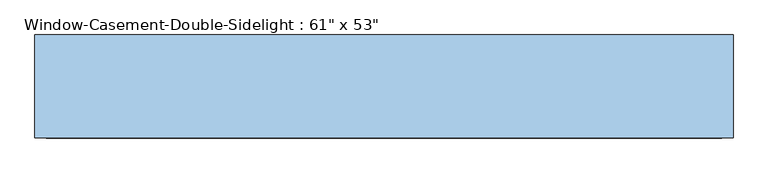
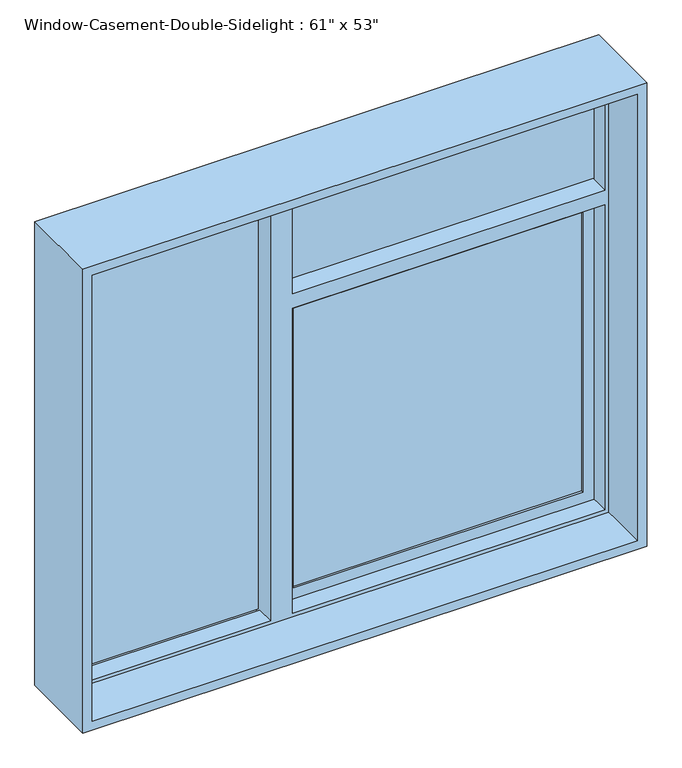
"""IFC4 building model written with IfcOpenShell, lengths in millimetres: window geometry."""

from ifc_helpers import new_model, si_unit, frame, origin, place, context, project, spatial, polyline, outline, extrude, faceted_brep, source, transform, mapped, element, save


def window_390faff0(model_context):
    return source(origin(), model_context, "Body", "SolidModel", [
        extrude(outline(polyline([(707.4296875, 98.425), (-87.6696875, 98.425), (-87.6696875, 111.125), (707.4296875, 111.125), (707.4296875, 98.425)])), frame((0.0, 0.0, 981.6703125), z_axis=(0.0, 0.0, 1.0), x_axis=(1.0, 0.0, 0.0)), (0.0, 0.0, 1.0), 812.2642187),
        extrude(outline(polyline([(707.4296875, 85.725), (707.4296875, 79.375), (-87.6696875, 79.375), (-87.6696875, 85.725), (707.4296875, 85.725)])), frame((0.0, 0.0, 981.6703125), z_axis=(0.0, 0.0, 1.0), x_axis=(1.0, 0.0, 0.0)), (0.0, 0.0, 1.0), 812.2642187),
        extrude(outline(polyline([(-180.34, 98.425), (-180.34, 92.075), (-749.3, 92.075), (-749.3, 98.425), (-180.34, 98.425)])), frame((0.0, 0.0, 949.9203125), z_axis=(0.0, 0.0, 1.0), x_axis=(1.0, 0.0, 0.0)), (0.0, 0.0, 1.0), 1285.2796875),
        extrude(outline(polyline([(-180.34, 85.725), (-180.34, 79.375), (-749.3, 79.375), (-749.3, 85.725), (-180.34, 85.725)])), frame((0.0, 0.0, 949.9203125), z_axis=(0.0, 0.0, 1.0), x_axis=(1.0, 0.0, 0.0)), (0.0, 0.0, 1.0), 1285.2796875),
        extrude(outline(polyline([(749.3, 85.725), (749.3, 79.375), (-129.54, 79.375), (-129.54, 85.725), (749.3, 85.725)])), frame((0.0, 0.0, 1877.6751563), z_axis=(0.0, 0.0, 1.0), x_axis=(1.0, 0.0, 0.0)), (0.0, 0.0, 1.0), 357.5248438),
        extrude(outline(polyline([(749.3, 98.425), (749.3, 92.075), (-129.54, 92.075), (-129.54, 98.425), (749.3, 98.425)])), frame((0.0, 0.0, 1877.6751563), z_axis=(0.0, 0.0, 1.0), x_axis=(1.0, 0.0, 0.0)), (0.0, 0.0, 1.0), 357.5248438),
        faceted_brep([(-749.3, 73.025, 2235.2), (-749.3, 114.3, 2235.2), (749.3, 114.3, 2235.2), (749.3, 73.025, 2235.2), (-129.54, 73.025, 2235.2), (-129.54, 111.125, 2235.2), (-180.34, 111.125, 2235.2), (-180.34, 73.025, 2235.2), (-739.1796875, 22.225, 2225.0796875), (-739.1796875, 73.025, 2225.0796875), (-180.34, 73.025, 2225.0796875), (-180.34, 22.225, 2225.0796875), (739.1796875, 73.025, 2225.0796875), (739.1796875, 22.225, 2225.0796875), (-119.4196875, 22.225, 2225.0796875), (-119.4196875, 73.025, 2225.0796875), (-749.3, -114.3, 2235.2), (-749.3, 22.225, 2235.2), (749.3, 22.225, 2235.2), (749.3, -114.3, 2235.2), (-774.7, 114.3, 2260.6), (-774.7, -114.3, 2260.6), (774.7, -114.3, 2260.6), (774.7, 114.3, 2260.6), (749.3, 114.3, 939.8), (749.3, 73.025, 939.8), (749.3, 73.025, 1835.8048438), (749.3, 111.125, 1835.8048438), (749.3, 111.125, 1877.6751563), (749.3, 73.025, 1877.6751563), (739.1796875, 73.025, 1877.6751563), (739.1796875, 22.225, 1877.6751563), (739.1796875, 73.025, 949.9203125), (739.1796875, 22.225, 949.9203125), (739.1796875, 22.225, 1835.8048438), (739.1796875, 73.025, 1835.8048438), (749.3, 22.225, 939.8), (749.3, -114.3, 939.8), (774.7, -114.3, 914.4), (774.7, 114.3, 914.4), (-749.3, 114.3, 939.8), (-749.3, 73.025, 939.8), (-180.34, 73.025, 939.8), (-180.34, 111.125, 939.8), (-129.54, 111.125, 939.8), (-129.54, 73.025, 939.8), (-119.4196875, 73.025, 949.9203125), (-119.4196875, 22.225, 949.9203125), (-739.1796875, 73.025, 949.9203125), (-739.1796875, 22.225, 949.9203125), (-180.34, 22.225, 949.9203125), (-180.34, 73.025, 949.9203125), (-749.3, 22.225, 939.8), (-749.3, -114.3, 939.8), (-774.7, -114.3, 914.4), (-774.7, 114.3, 914.4), (-119.4196875, 73.025, 1877.6751563), (-129.54, 73.025, 1877.6751563), (-129.54, 73.025, 1835.8048438), (-119.4196875, 73.025, 1835.8048438), (-119.4196875, 22.225, 1877.6751563), (-119.4196875, 22.225, 1835.8048438), (-129.54, 111.125, 1877.6751563), (-129.54, 111.125, 1835.8048438)], [[[0, 1, 2, 3, 4, 5, 6, 7]], [[8, 9, 10, 11]], [[12, 13, 14, 15]], [[16, 17, 18, 19]], [[20, 21, 22, 23]], [[3, 2, 24, 25, 26, 27, 28, 29]], [[13, 12, 30, 31]], [[32, 33, 34, 35]], [[19, 18, 36, 37]], [[23, 22, 38, 39]], [[25, 24, 40, 41, 42, 43, 44, 45]], [[33, 32, 46, 47]], [[48, 49, 50, 51]], [[37, 36, 52, 53]], [[39, 38, 54, 55]], [[1, 0, 41, 40]], [[12, 15, 56, 57, 4, 3, 29, 30]], [[46, 32, 35, 26, 25, 45, 58, 59]], [[41, 0, 7, 10, 9, 48, 51, 42]], [[9, 8, 49, 48]], [[17, 52, 36, 18], [13, 31, 60, 14], [33, 47, 61, 34], [49, 8, 11, 50]], [[17, 16, 53, 52]], [[22, 21, 54, 38], [16, 19, 37, 53]], [[21, 20, 55, 54]], [[20, 23, 39, 55], [2, 1, 40, 24]], [[43, 6, 5, 62, 28, 27, 63, 44]], [[6, 43, 42, 51, 50, 11, 10, 7]], [[15, 14, 60, 56]], [[47, 46, 59, 61]], [[5, 4, 57, 62]], [[45, 44, 63, 58]], [[63, 27, 26, 35, 34, 61, 59, 58]], [[28, 62, 57, 56, 60, 31, 30, 29]]]),
        extrude(outline(polyline([(1835.8048438, 749.3), (1835.8048438, -129.54), (939.8, -129.54), (939.8, 749.3), (1835.8048438, 749.3)]), holes=[polyline([(981.6703125, 707.4296875), (981.6703125, -87.6696875), (1793.9345313, -87.6696875), (1793.9345313, 707.4296875), (981.6703125, 707.4296875)])]), frame((0.0, 73.025, 0.0), z_axis=(0.0, 1.0, 0.0), x_axis=(0.0, 0.0, 1.0)), (0.0, 0.0, 1.0), 31.75),
    ])


if __name__ == "__main__":
    model = new_model("IFC4")
    model_context = context("Model", 3, world=origin())
    ifc_project = project(units=[si_unit("LENGTHUNIT", "METRE", prefix="MILLI")], contexts=[model_context])
    site = spatial("IfcSite", under=ifc_project)
    building = spatial("IfcBuilding", under=site)
    placement = place(None, origin())
    window_shape = window_390faff0(model_context)
    element("IfcWindow", 1, ObjectType="Window-Casement-Double-Sidelight : 61\" x 53\"", at=placement, inside=building, context=model_context, shape_type="MappedRepresentation", body=[
        mapped(window_shape, transform((0.0, 0.0, 0.0), x_axis=(1.0, 0.0, 0.0), y_axis=(0.0, 1.0, 0.0), z_axis=(0.0, 0.0, 1.0))),
    ])
    save(model, "model.ifc")

# Revit data of these elements
# Type "Window-Casement-Double-Sidelight : 61\" x 53\""
#   Type Mark = "21"
#   Fire Rating = "0.5h"
#   Assembly Code = "B2020100"
#   Analytic Construction = "Double glazing - domestic"
#   Window Inset [instance default] = 0' - 0 5/8"
#   Wall Thickness [instance default] = 0' - 6"
#   Visual Light Transmittance = 0.81
#   Transom Height Ratio = 0.3
#   Transom Height = 1' - 3.9"
#   Thermal Resistance (R) = 1.8146 (h·ft²·°F)/BTU
#   Solar Heat Gain Coefficient = 0.76
#   Side Width = 2' - 0.4"
#   Rough Width = 5' - 1 1/2"
#   Rough Height = 4' - 5 1/2"
#   Opening Window Width = 3' - 0.6"
#   Opening Window Height = 3' - 1.1"
#   Heat Transfer Coefficient (U) = 0.5511 BTU/(h·ft²·°F)
#   Height = 4' - 5"
#   Frame Gap 3 [instance default] = 0' - 1 83/128"
#   Frame Gap 2 [instance default] = 0' - 0 5/8"
#   Frame Gap 1 = 0' - 1 51/128"
#   Default Sill Height = 3' - 0"
#   Width = 5' - 1"
#   Frame Material = Metal - Aluminum
#   Glass Panel Material = Glass
#   Wall Closure = (empty or 0)
# Element 1 (IfcWindow, "Window-Casement-Double-Sidelight : 61\" x 53\"")
#   Wall Thickness = 0' - 9"
#   Materials on its faces: "Metal - Aluminum", "Glass"
# Materials
#   "Metal - Aluminum": class "Metal", colour RGB 247 247 247, transparency 0
#   "Glass": class "Glass", colour RGB 0 128 192, transparency 0.75, Description = "Soda Lime Glass", Cost = 0
